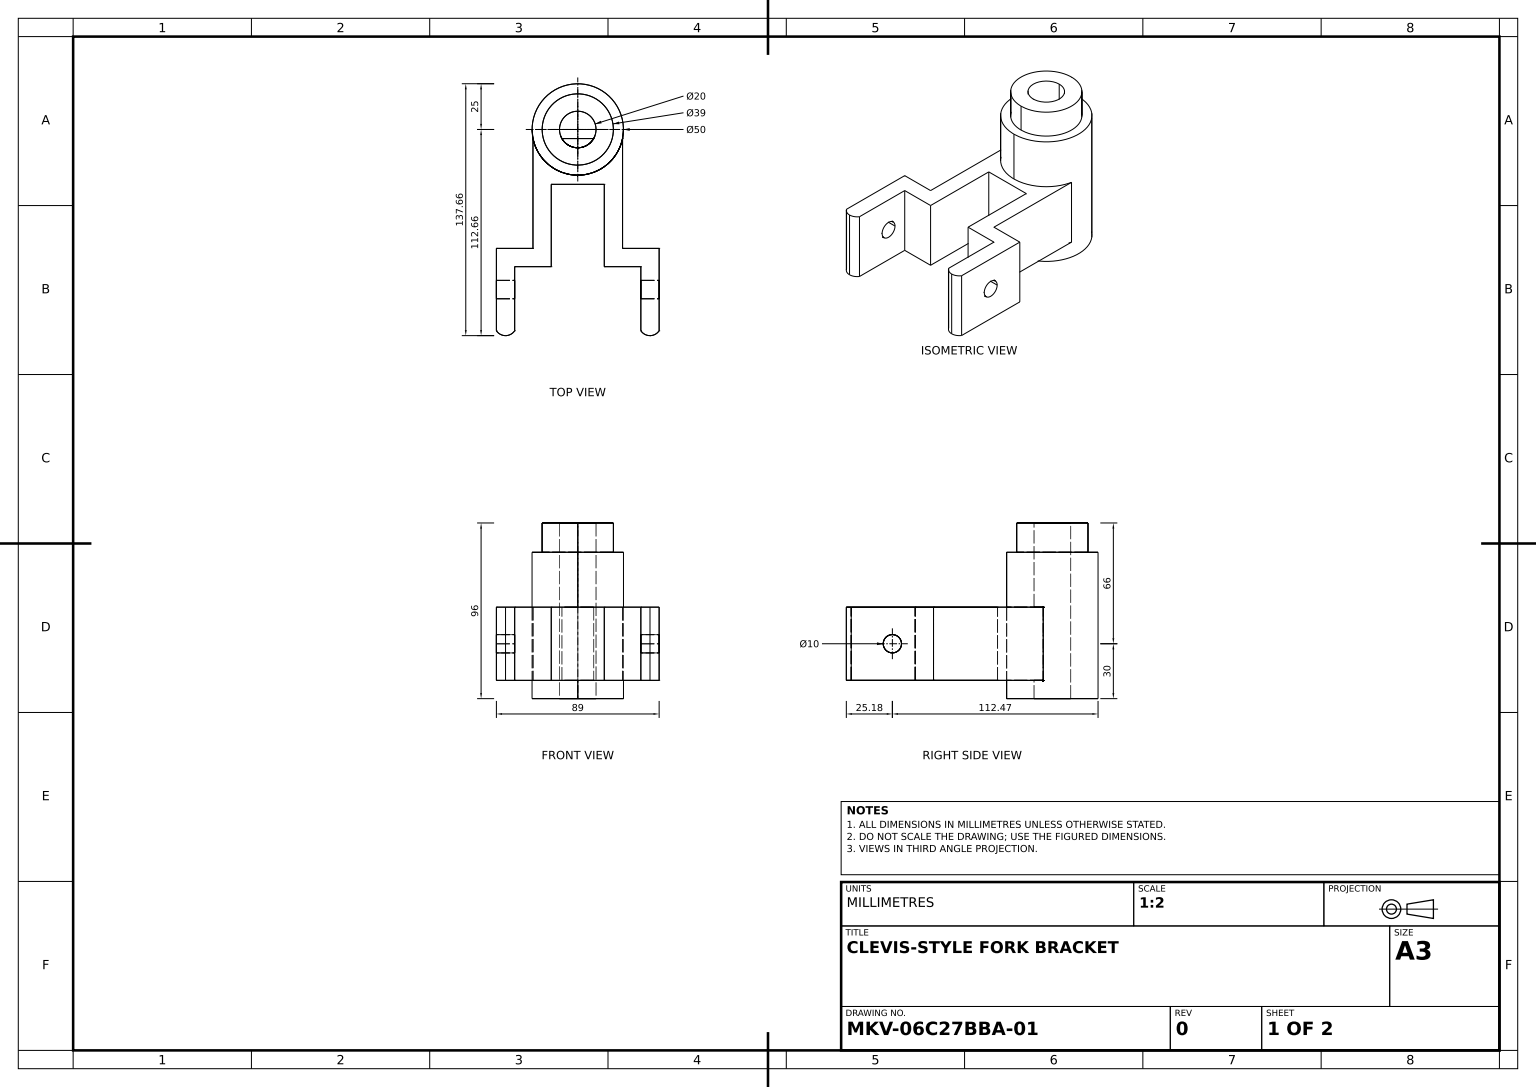
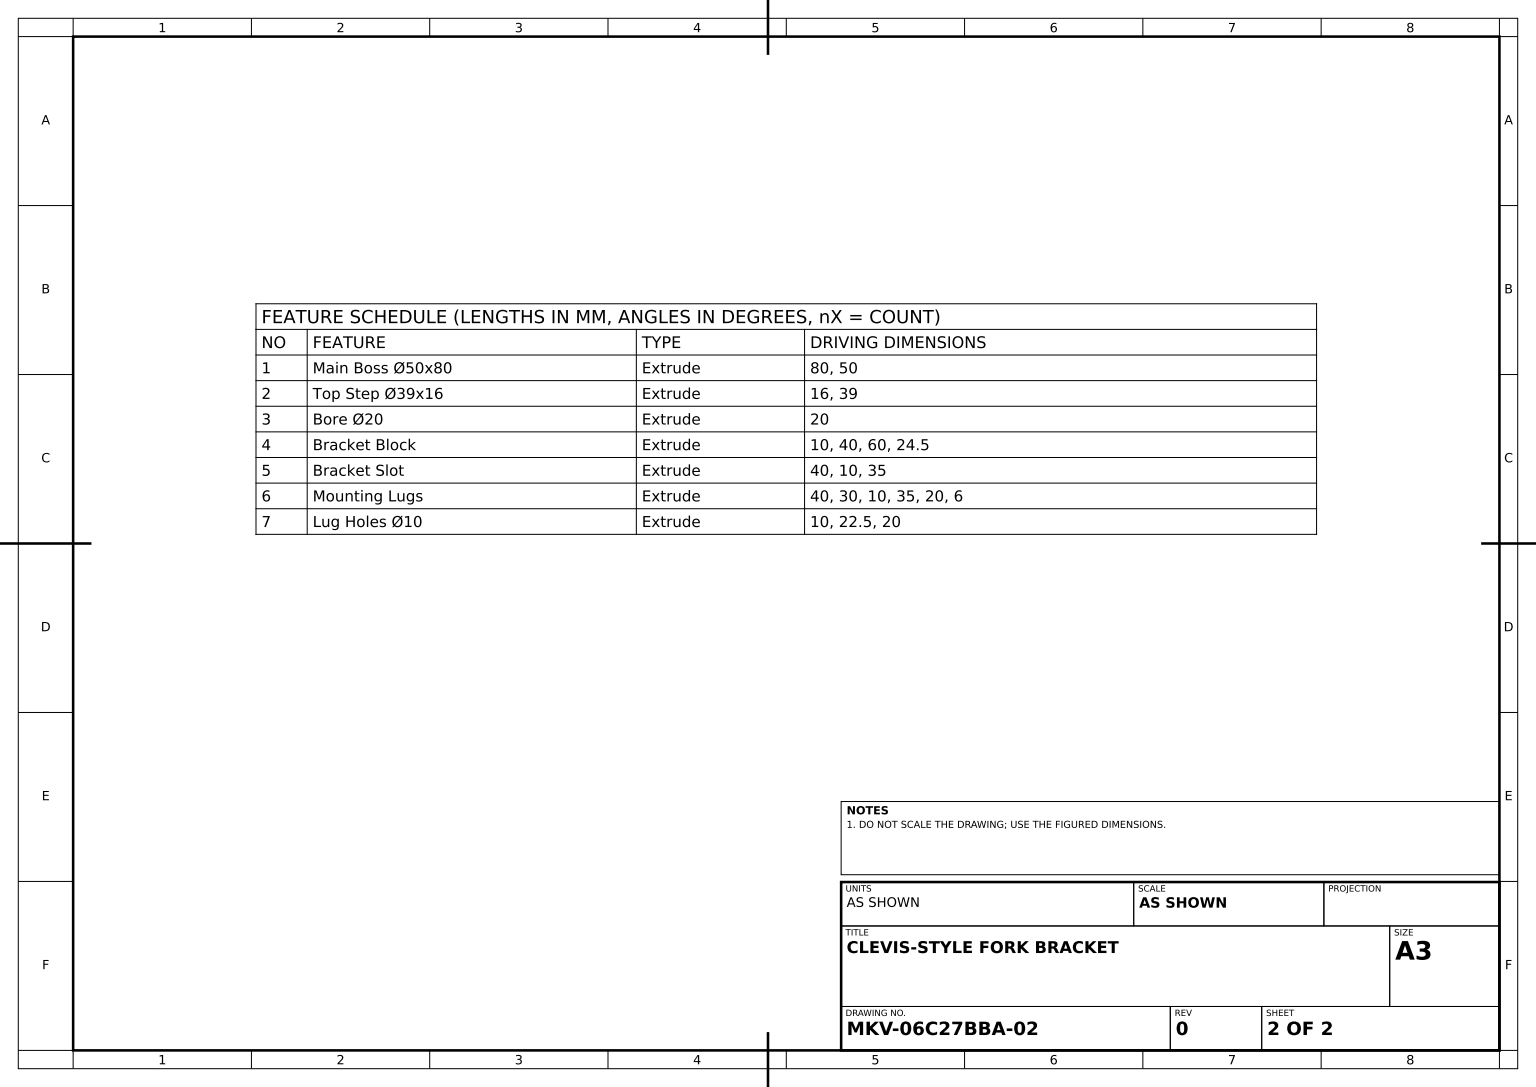
from build123d import *

# Parameters (mm, degrees)
MAIN_BOSS_SKETCH_50_R  = 25
MAIN_BOSS_50X80_DEPTH  = 80
TOP_STEP_SKETCH_39_R   = 19.5
TOP_STEP_39X16_DEPTH   = 16
BORE_SKETCH_20_R       = 10
BORE_20_DEPTH          = 103.303470127
BRACKET_BLOCK_SKETCH_W = 49
BRACKET_BLOCK_SKETCH_H = 60
BRACKET_BLOCK_DEPTH    = 40
BRACKET_SLOT_SKETCH_W  = 29
BRACKET_SLOT_SKETCH_H  = 35
BRACKET_SLOT_DEPTH     = 40
MOUNTING_LUGS_DEPTH    = 40
LUG_HOLE_SKETCH_10_R   = 5
LUG_HOLES_10_DEPTH     = 173.710437877


with BuildPart() as part:
    # Main Boss Sketch Ø50 → Main Boss Ø50x80 (new body)
    with BuildSketch(Plane(origin=(0, 0, 0), x_dir=(1, 0, 0), z_dir=(0, 1, 0))):
        with Locations(Location((0, 0, 0), (0, 0, 270))):
            Circle(MAIN_BOSS_SKETCH_50_R)
    extrude(amount=MAIN_BOSS_50X80_DEPTH)

    # Top Step Sketch Ø39 → Top Step Ø39x16 (add)
    with BuildSketch(Plane(origin=(0, 80, 0), x_dir=(1, 0, 0), z_dir=(0, 1, 0))):
        with Locations(Location((0, 0, 0), (0, 0, 270))):
            Circle(TOP_STEP_SKETCH_39_R)
    extrude(amount=TOP_STEP_39X16_DEPTH)

    # Bore Sketch Ø20 → Bore Ø20 (cut, through all)
    with BuildSketch(Plane(origin=(0, 96, 0), x_dir=(1, 0, 0), z_dir=(0, 1, 0))):
        with Locations(Location((0, 0, 0), (0, 0, 270))):
            Circle(BORE_SKETCH_20_R)
    extrude(amount=-BORE_20_DEPTH, mode=Mode.SUBTRACT)

    # Bracket Block Sketch → Bracket Block (add)
    with BuildSketch(Plane(origin=(0, 10, 0), x_dir=(1, 0, 0), z_dir=(0, 1, 0))):
        with Locations((0, -34.974937186)):
            Rectangle(BRACKET_BLOCK_SKETCH_W, BRACKET_BLOCK_SKETCH_H)
    extrude(amount=BRACKET_BLOCK_DEPTH)

    # Bracket Slot Sketch → Bracket Slot (cut)
    with BuildSketch(Plane(origin=(0, 50, 0), x_dir=(1, 0, 0), z_dir=(0, 1, 0))):
        with Locations((0, -47.474937186)):
            Rectangle(BRACKET_SLOT_SKETCH_W, BRACKET_SLOT_SKETCH_H)
    extrude(amount=-BRACKET_SLOT_DEPTH, mode=Mode.SUBTRACT)

    # Mounting Lugs Sketch → Mounting Lugs (add)
    with BuildSketch(Plane(origin=(0, 50, 0), x_dir=(1, 0, 0), z_dir=(0, 1, 0))):
        with BuildLine():
            Line((14.5, -64.974937186), (44.5, -64.974937186))
            Line((44.5, -64.974937186), (44.5, -74.974937186))
            Line((44.5, -74.974937186), (44.5, -109.974937186))
            ThreePointArc((44.5, -109.974937186), (39.5, -112.658312395), (34.5, -109.974937186))
            Line((34.5, -109.974937186), (34.5, -74.974937186))
            Line((34.5, -74.974937186), (14.5, -74.974937186))
            Line((14.5, -74.974937186), (14.5, -64.974937186))
        make_face()
        with BuildLine():
            Line((-14.5, -64.974937186), (-44.5, -64.974937186))
            Line((-44.5, -64.974937186), (-44.5, -74.974937186))
            Line((-44.5, -74.974937186), (-44.5, -109.974937186))
            ThreePointArc((-44.5, -109.974937186), (-39.5, -112.658312395), (-34.5, -109.974937186))
            Line((-34.5, -109.974937186), (-34.5, -74.974937186))
            Line((-34.5, -74.974937186), (-14.5, -74.974937186))
            Line((-14.5, -74.974937186), (-14.5, -64.974937186))
        make_face()
    extrude(amount=-MOUNTING_LUGS_DEPTH)

    # Lug Hole Sketch Ø10 → Lug Holes Ø10 (cut, through all)
    with BuildSketch(Plane(origin=(44.5, 0, 0), x_dir=(0, 0, -1), z_dir=(1, 0, 0))):
        with Locations((-87.474937186, 30)):
            Circle(LUG_HOLE_SKETCH_10_R)
    extrude(amount=-LUG_HOLES_10_DEPTH, mode=Mode.SUBTRACT)


solid = part.part
